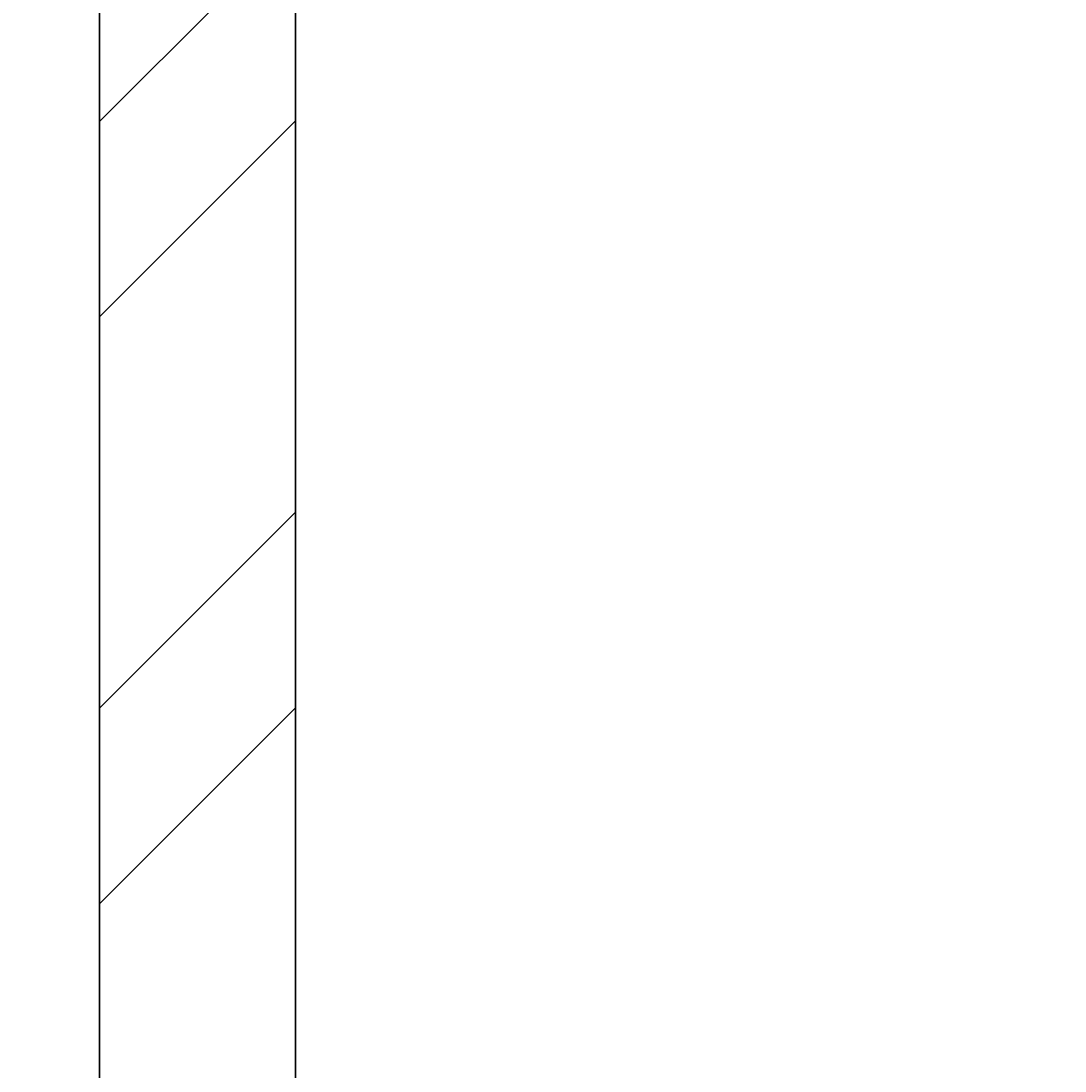
# Model space of a CAD drawing. Units: inches. Extents: x 1885 to 2748, y 783 to 2421.
# Tile 7 of 117: x 1969 to 1993, y 1114 to 1138. Entities that reach past the tile are written whole.
import ezdxf

# ---------------------------------------------------------------- set-up
doc = ezdxf.new("R2010")
doc.units = ezdxf.units.IN
doc.layers.add('A-ANNO-DIMS', color=2, linetype='Continuous', lineweight=18)
doc.layers.add('A-WALL', color=7, linetype='Continuous', lineweight=35)
doc.layers.add('A-WALL-PATT', color=85, linetype='Continuous', lineweight=13, true_color=0x58ba48)
doc.styles.get("Standard").update_dxf_attribs({"font": 'arial.ttf'})
doc.dimstyles.get("Standard").update_dxf_attribs({"dimtxt": 0.18, "dimasz": 0.18, "dimexe": 0.18, "dimexo": 0.0625, "dimgap": 0.09, "dimtad": 0, "dimtih": 1, "dimtoh": 1, "dimdec": 4, "dimzin": 0, "dimdsep": 46, "dimtxsty": 'Standard', "dimcen": 0.09, "dimadec": 0, "dimazin": 0, "dimtfac": 1, "dimtdec": 4, "dimtofl": 0, "dimtmove": 0, "dimatfit": 3, "dimfxl": 1, "dimtolj": 1, "dimtzin": 0, "dimarcsym": 0})

# ---------------------------------------------------------------- blocks, each defined once
blk = doc.blocks.new('*D45')
at = {"layer": 'A-ANNO-DIMS', "color": 0, "lineweight": -2, "transparency": 16777216}
for p, q in [((1980.711, 1524.006), (1902.844, 1524.006)), ((1903.024, 1523.826), (1903.024, 1290.937)), ((1903.024, 1057.686), (1903.024, 1290.574)), ((1971.211, 1057.506), (1902.844, 1057.506))]:
    blk.add_line(p, q, dxfattribs=at)
at = {"layer": 'A-ANNO-DIMS', "color": 0, "transparency": 16777216}
for points in [[(1902.994, 1523.826), (1903.054, 1523.826), (1903.024, 1524.006)], [(1902.994, 1057.686), (1903.054, 1057.686), (1903.024, 1057.506)]]:
    blk.add_solid(points, dxfattribs=at)
at = {"layer": 'Defpoints', "color": 0, "transparency": 16777216}
for p in [(1903.024, 1524.006), (1980.774, 1524.006), (1971.274, 1057.506)]:
    blk.add_point(p, dxfattribs=at)
at = {"layer": 'A-ANNO-DIMS', "color": 0, "transparency": 16777216, "insert": (1903.024, 1290.756), "char_height": 0.18, "attachment_point": 5}
blk.add_mtext('\\A1;466.5', dxfattribs=at)

msp = doc.modelspace()

# ---------------------------------------------------------------- hatches: boundary and pattern name
at = {"layer": 'A-WALL-PATT'}
h = msp.add_hatch(dxfattribs=at)
h.set_pattern_fill('ANSI32', color=256)
h.paths.add_polyline_path([(2007.772, 2318.006), (1980.774, 2318.006), (1980.774, 2281.215), (1985.274, 2281.215), (1985.274, 2313.506), (2007.772, 2313.506), (2007.772, 2315.756)])
h.paths.add_polyline_path([(2094.324, 2318.006), (2067.772, 2318.006), (2067.772, 2313.506), (2094.324, 2313.506), (2094.324, 2315.756)])
h.paths.add_polyline_path([(2131.367, 2315.756), (2131.367, 2318.006), (2131.189, 2318.006), (2112.609, 2318.006), (2112.609, 2313.506), (2117.274, 2313.506), (2117.274, 2255.201), (2121.774, 2255.201), (2121.774, 2313.506), (2131.367, 2313.506)])
h.paths.add_polyline_path([(2190.512, 2318.006), (2155.367, 2318.006), (2155.367, 2313.506), (2169.774, 2313.506), (2169.774, 2229.506), (2121.774, 2229.506), (2121.774, 2233.451), (2119.524, 2233.451), (2117.274, 2233.451), (2117.274, 2201.101), (2121.774, 2201.101), (2121.774, 2225.006), (2169.774, 2225.006), (2169.774, 2165.006), (2306.274, 2165.006), (2306.274, 2066.006), (2310.774, 2066.006), (2344.274, 2066.006), (2486.274, 2066.006), (2486.274, 1886.006), (2483.02, 1886.006), (2483.02, 1881.506), (2486.274, 1881.506), (2486.274, 1880.678), (2490.774, 1880.678), (2490.774, 2070.506), (2344.274, 2070.506), (2310.774, 2070.506), (2310.774, 2165.006), (2310.774, 2173.636), (2308.524, 2173.636), (2306.274, 2173.636), (2306.274, 2169.506), (2174.274, 2169.506), (2174.274, 2313.506), (2190.512, 2313.506), (2190.512, 2315.756)])
h.paths.add_polyline_path([(1985.274, 2221.215), (1980.774, 2221.215), (1980.774, 2165.006), (1992.774, 2165.006), (1992.774, 2141.927), (1997.274, 2141.927), (1997.274, 2165.006), (2117.274, 2165.006), (2117.274, 2163.126), (2121.774, 2163.126), (2121.774, 2172.734), (2119.524, 2172.734), (2117.274, 2172.734), (2117.274, 2169.506), (1985.274, 2169.506)])
h.paths.add_polyline_path([(1997.274, 2105.927), (1992.774, 2105.927), (1992.774, 2070.506), (2016.774, 2070.506), (2016.774, 2059.123), (2019.024, 2059.123), (2021.274, 2059.123), (2021.274, 2070.506), (2117.274, 2070.506), (2117.274, 2022.506), (2114.423, 2022.506), (2114.423, 2018.006), (2123.627, 2018.006), (2123.627, 2020.256), (2123.627, 2022.506), (2121.774, 2022.506), (2121.774, 2142.587), (2119.524, 2142.587), (2117.274, 2142.587), (2117.274, 2075.006), (1997.274, 2075.006)])
h.paths.add_polyline_path([(2092.029, 2020.256), (2092.029, 2022.506), (2021.274, 2022.506), (2021.274, 2035.123), (2016.774, 2035.123), (2016.774, 2018.006), (2016.774, 1978.784), (2021.274, 1978.784), (2021.274, 2018.006), (2092.029, 2018.006)])
h.paths.add_polyline_path([(2260.938, 2022.506), (2153.105, 2022.506), (2153.105, 2020.256), (2153.105, 2018.006), (2155.274, 2018.006), (2155.274, 1886.006), (2107.629, 1886.006), (2107.629, 1881.506), (2182.911, 1881.506), (2182.911, 1883.756), (2182.911, 1886.006), (2159.774, 1886.006), (2159.774, 2018.006), (2260.938, 2018.006), (2260.938, 2020.256)])
h.paths.add_polyline_path([(2047.629, 1883.756), (2047.629, 1886.006), (2021.274, 1886.006), (2021.274, 1918.784), (2019.024, 1918.784), (2016.774, 1918.784), (2016.774, 1881.506), (2047.629, 1881.506)])
h.paths.add_polyline_path([(2306.361, 1883.756), (2306.361, 1886.006), (2296.274, 1886.006), (2296.274, 1982.006), (2316.535, 1982.006), (2316.535, 1984.256), (2316.535, 1986.506), (2296.274, 1986.506), (2296.274, 2022.506), (2289.276, 2022.506), (2289.276, 2018.006), (2291.774, 2018.006), (2291.774, 1886.006), (2242.911, 1886.006), (2242.911, 1881.506), (2306.361, 1881.506)], flags=17)
h.paths.add_polyline_path([(1985.274, 1843.006), (2021.6, 1843.006), (2021.534, 1845.441), (2021.477, 1847.506), (1980.774, 1847.506), (1980.774, 1809.446), (1985.274, 1809.446)])
h.paths.add_polyline_path([(2131.482, 1845.256), (2131.482, 1847.506), (2081.534, 1847.506), (2081.534, 1843.006), (2117.274, 1843.006), (2117.274, 1784.147), (2119.524, 1784.147), (2121.774, 1784.147), (2121.774, 1843.006), (2131.482, 1843.006)])
h.paths.add_polyline_path([(2203.886, 1847.506), (2155.482, 1847.506), (2155.482, 1843.006), (2169.774, 1843.006), (2169.774, 1759.006), (2121.774, 1759.006), (2121.774, 1761.457), (2117.274, 1761.457), (2117.274, 1730.429), (2121.774, 1730.429), (2121.774, 1754.506), (2177.421, 1754.506), (2177.421, 1756.756), (2177.421, 1759.006), (2174.274, 1759.006), (2174.274, 1843.006), (2203.886, 1843.006)])
h.paths.add_polyline_path([(2335.554, 1845.256), (2335.554, 1847.506), (2239.886, 1847.506), (2239.886, 1843.006), (2306.274, 1843.006), (2306.274, 1759.006), (2199.486, 1759.006), (2199.486, 1754.506), (2310.774, 1754.506), (2310.774, 1843.006), (2335.554, 1843.006)])
h.paths.add_polyline_path([(2348.774, 2022.506), (2344.274, 2022.506), (2344.274, 1986.506), (2341.681, 1986.506), (2341.681, 1982.006), (2344.274, 1982.006), (2344.274, 1886.006), (2330.361, 1886.006), (2330.361, 1881.506), (2361.627, 1881.506), (2361.627, 1883.756), (2361.627, 1886.006), (2348.774, 1886.006)], flags=17)
h.paths.add_polyline_path([(2283.251, 2315.756), (2283.251, 2318.006), (2238.512, 2318.006), (2238.512, 2313.506), (2283.251, 2313.506)], flags=17)
h.paths.add_polyline_path([(2363.274, 2348.006), (2388.677, 2348.006), (2388.677, 2350.256), (2388.677, 2352.506), (2358.774, 2352.506), (2358.774, 2348.006), (2358.774, 2318.006), (2344.481, 2318.006), (2344.481, 2313.506), (2358.774, 2313.506), (2358.774, 2229.506), (2310.774, 2229.506), (2310.774, 2231.952), (2306.274, 2231.952), (2306.274, 2205.611), (2310.774, 2205.611), (2310.774, 2225.006), (2358.774, 2225.006), (2358.774, 2211.506), (2452.329, 2211.506), (2452.329, 2213.756), (2452.329, 2216.006), (2363.274, 2216.006), (2363.274, 2318.006)])
h.paths.add_polyline_path([(2310.774, 2313.506), (2320.481, 2313.506), (2320.481, 2315.756), (2320.481, 2318.006), (2302.728, 2318.006), (2302.728, 2313.506), (2306.274, 2313.506), (2306.274, 2251.076), (2310.774, 2251.076)], flags=17)
h.paths.add_polyline_path([(2490.774, 2352.506), (2486.274, 2352.506), (2448.677, 2352.506), (2448.677, 2348.006), (2486.274, 2348.006), (2486.274, 2318.006), (2486.274, 2216.006), (2481.78, 2216.006), (2481.78, 2211.506), (2486.274, 2211.506), (2486.274, 2165.006), (2493.289, 2165.006), (2493.289, 2167.256), (2493.289, 2169.506), (2490.774, 2169.506), (2490.774, 2313.506), (2494.429, 2313.506), (2494.429, 2318.006), (2490.774, 2318.006)])
h.paths.add_polyline_path([(2534.653, 2318.006), (2515.691, 2318.006), (2515.691, 2313.506), (2534.653, 2313.506), (2534.653, 2315.756)])
h.paths.add_polyline_path([(2618.274, 2318.006), (2594.653, 2318.006), (2594.653, 2313.506), (2613.774, 2313.506), (2613.774, 2281.706), (2618.274, 2281.706)])
h.paths.add_polyline_path([(2618.274, 2221.706), (2613.774, 2221.706), (2613.774, 2169.506), (2554.019, 2169.506), (2554.019, 2165.006), (2613.774, 2165.006), (2613.774, 2152.878), (2618.274, 2152.878)])
h.paths.add_polyline_path([(2618.274, 2128.878), (2616.024, 2128.878), (2613.774, 2128.878), (2613.774, 2117.006), (2529.774, 2117.006), (2529.774, 2165.006), (2532.848, 2165.006), (2532.848, 2169.506), (2522.867, 2169.506), (2522.867, 2165.006), (2525.274, 2165.006), (2525.274, 2117.006), (2525.274, 2112.506), (2525.274, 2108.576), (2529.774, 2108.576), (2529.774, 2112.506), (2613.774, 2112.506), (2613.774, 2080.19), (2618.274, 2080.19)])
h.paths.add_polyline_path([(2618.274, 2044.19), (2616.024, 2044.19), (2613.774, 2044.19), (2613.774, 2015.506), (2529.774, 2015.506), (2529.774, 2088.582), (2527.524, 2088.582), (2525.274, 2088.582), (2525.274, 2011.006), (2613.774, 2011.006), (2613.774, 1956.755), (2618.274, 1956.755)])
h.paths.add_polyline_path([(2618.274, 1881.506), (2618.274, 1896.755), (2613.774, 1896.755), (2613.774, 1881.506), (2613.774, 1847.506), (2592.715, 1847.506), (2592.715, 1843.006), (2613.774, 1843.006), (2613.774, 1765.006), (2613.774, 1760.506), (2609.621, 1760.506), (2609.621, 1756.006), (2613.774, 1756.006), (2613.774, 1660.006), (2608.544, 1660.006), (2608.544, 1655.506), (2613.774, 1655.506), (2613.774, 1508.158), (2618.274, 1508.158)])
h.paths.add_polyline_path([(2565.774, 1843.006), (2568.997, 1843.006), (2568.997, 1847.506), (2490.774, 1847.506), (2490.774, 1849.7), (2488.524, 1849.7), (2486.274, 1849.7), (2486.274, 1847.506), (2477.274, 1847.506), (2477.274, 1838.506), (2477.274, 1821.493), (2486.274, 1821.493), (2486.274, 1838.506), (2561.274, 1838.506), (2561.274, 1765.006), (2486.274, 1765.006), (2486.274, 1786.157), (2477.274, 1786.157), (2477.274, 1765.006), (2477.274, 1756.006), (2486.274, 1756.006), (2565.774, 1756.006), (2585.621, 1756.006), (2585.621, 1758.256), (2585.621, 1760.506), (2565.774, 1760.506), (2565.774, 1765.006)])
h.paths.add_polyline_path([(2486.274, 1651.006), (2561.274, 1651.006), (2561.274, 1567.006), (2486.274, 1567.006), (2486.274, 1591.321), (2477.274, 1591.321), (2477.274, 1567.006), (2477.274, 1558.006), (2477.274, 1555.439), (2481.774, 1555.439), (2481.774, 1558.006), (2568.653, 1558.006), (2568.653, 1560.256), (2568.653, 1562.506), (2565.774, 1562.506), (2565.774, 1655.506), (2584.544, 1655.506), (2584.544, 1657.756), (2584.544, 1660.006), (2565.774, 1660.006), (2486.274, 1660.006), (2477.274, 1660.006), (2477.274, 1651.006), (2477.274, 1632.989), (2486.274, 1632.989)])
h.paths.add_polyline_path([(2449.967, 1883.756), (2449.967, 1886.006), (2421.627, 1886.006), (2421.627, 1881.506), (2449.967, 1881.506)], flags=17)
h.paths.add_polyline_path([(2447.274, 1847.506), (2395.554, 1847.506), (2395.554, 1843.006), (2442.774, 1843.006), (2442.774, 1809.27), (2447.274, 1809.27)])
h.paths.add_polyline_path([(1985.274, 1749.446), (1980.774, 1749.446), (1980.774, 1694.504), (1985.274, 1694.504), (1985.274, 1694.506), (1986.897, 1694.506), (1986.897, 1697.78), (1986.897, 1699.006), (1985.274, 1699.006)])
h.paths.add_polyline_path([(2152.774, 1699.006), (2121.774, 1699.006), (2121.774, 1703.668), (2119.524, 1703.668), (2117.274, 1703.668), (2117.274, 1699.006), (2009.219, 1699.006), (2009.219, 1694.506), (2148.274, 1694.506), (2148.274, 1692.631), (2152.774, 1692.631)])
h.paths.add_polyline_path([(2016.274, 1694.506), (2011.774, 1694.506), (2011.774, 1558.006), (2040.806, 1558.006), (2040.806, 1560.256), (2040.806, 1562.506), (2016.274, 1562.506)])
h.paths.add_polyline_path([(2152.774, 1663.017), (2150.524, 1663.017), (2148.274, 1663.017), (2148.274, 1562.506), (2100.806, 1562.506), (2100.806, 1558.006), (2165.119, 1558.006), (2165.119, 1560.256), (2165.119, 1562.506), (2152.774, 1562.506), (2152.774, 1610.506), (2224.774, 1610.506), (2224.774, 1607.99), (2229.274, 1607.99), (2229.274, 1615.006), (2152.774, 1615.006)])
h.paths.add_polyline_path([(2238.613, 1560.256), (2238.613, 1562.506), (2229.274, 1562.506), (2229.274, 1588.756), (2227.024, 1588.763), (2224.774, 1588.771), (2224.774, 1562.506), (2189.119, 1562.506), (2189.119, 1558.006), (2238.613, 1558.006)])
h.paths.add_polyline_path([(2336.024, 1560.256), (2336.024, 1562.506), (2310.774, 1562.506), (2310.774, 1656.347), (2308.524, 1656.347), (2306.274, 1656.347), (2306.274, 1562.506), (2286.613, 1562.506), (2286.613, 1558.006), (2336.024, 1558.006)])
h.paths.add_polyline_path([(2447.274, 1690.968), (2445.024, 1690.968), (2442.774, 1690.968), (2442.774, 1687.006), (2306.274, 1687.006), (2306.274, 1680.75), (2310.774, 1680.75), (2310.774, 1682.506), (2442.774, 1682.506), (2442.774, 1562.506), (2396.024, 1562.506), (2396.024, 1558.006), (2447.274, 1558.006)])
h.paths.add_polyline_path([(2447.274, 1749.27), (2445.024, 1749.27), (2442.774, 1749.27), (2442.774, 1717.232), (2447.274, 1717.232)])
h.paths.add_polyline_path([(2044.674, 1521.756), (2044.674, 1524.006), (2007.274, 1524.006), (2007.274, 1503.49), (2009.524, 1503.49), (2011.774, 1503.49), (2011.774, 1519.506), (2044.674, 1519.506)])
h.paths.add_polyline_path([(2177.969, 1521.756), (2177.969, 1524.006), (2104.674, 1524.006), (2104.674, 1519.506), (2145.774, 1519.506), (2145.774, 1387.506), (2143.37, 1387.506), (2143.37, 1383.006), (2251.585, 1383.006), (2251.585, 1385.256), (2251.585, 1387.506), (2150.274, 1387.506), (2150.274, 1519.506), (2177.969, 1519.506)])
h.paths.add_polyline_path([(2298.704, 1524.006), (2237.969, 1524.006), (2237.969, 1519.506), (2282.274, 1519.506), (2282.274, 1387.506), (2279.683, 1387.506), (2279.683, 1383.006), (2286.774, 1383.006), (2286.774, 1419.006), (2312.451, 1419.006), (2312.451, 1421.256), (2312.451, 1423.506), (2286.774, 1423.506), (2286.774, 1519.506), (2298.704, 1519.506), (2298.704, 1521.722)], flags=17)
h.paths.add_polyline_path([(2361.897, 1521.756), (2361.897, 1524.006), (2322.704, 1524.006), (2322.704, 1519.506), (2334.774, 1519.506), (2334.774, 1423.506), (2331.93, 1423.506), (2331.93, 1419.006), (2334.774, 1419.006), (2334.774, 1387.506), (2334.774, 1383.228), (2339.274, 1383.228), (2339.274, 1387.506), (2339.274, 1519.506), (2361.897, 1519.506)], flags=17)
h.paths.add_polyline_path([(2447.274, 1521.756), (2447.274, 1524.006), (2421.897, 1524.006), (2421.897, 1519.506), (2447.274, 1519.506)], flags=17)
h.paths.add_polyline_path([(2481.774, 1529.6), (2479.524, 1529.6), (2477.274, 1529.6), (2477.274, 1524.006), (2474.489, 1524.006), (2474.489, 1519.506), (2477.274, 1519.506), (2477.274, 1334.506), (2296.774, 1334.506), (2296.774, 1240.506), (2160.274, 1240.506), (2160.274, 1180.506), (2112.274, 1180.506), (2112.274, 1207.692), (2110.024, 1207.692), (2107.774, 1207.692), (2107.774, 1171.609), (2112.274, 1171.609), (2112.274, 1176.006), (2160.274, 1176.006), (2160.274, 1092.006), (2144.221, 1092.006), (2144.221, 1087.506), (2189.497, 1087.506), (2189.497, 1089.756), (2189.497, 1092.006), (2164.774, 1092.006), (2164.774, 1236.006), (2296.774, 1236.006), (2296.774, 1231.912), (2301.274, 1231.912), (2301.274, 1330.006), (2481.774, 1330.006), (2481.774, 1387.506)])
h.paths.add_polyline_path([(2618.274, 1448.158), (2613.774, 1448.158), (2613.774, 1382.506), (2529.774, 1382.506), (2525.274, 1382.506), (2525.274, 1307.062), (2529.774, 1307.062), (2529.774, 1378.006), (2613.774, 1378.006), (2613.774, 1354.988), (2618.274, 1354.988)])
h.paths.add_polyline_path([(2618.274, 1318.988), (2613.774, 1318.988), (2613.774, 1281.006), (2529.774, 1281.006), (2529.774, 1283.786), (2527.524, 1283.786), (2525.274, 1283.786), (2525.274, 1228.506), (2516.794, 1228.506), (2516.794, 1224.006), (2533.484, 1224.006), (2533.484, 1226.256), (2533.484, 1228.506), (2529.774, 1228.506), (2529.774, 1276.506), (2613.774, 1276.506), (2613.774, 1266.02), (2618.274, 1266.02)])
h.paths.add_polyline_path([(2618.274, 1134.964), (2613.774, 1134.964), (2613.774, 1092.006), (2594.545, 1092.006), (2594.545, 1087.506), (2618.274, 1087.506)])
h.paths.add_polyline_path([(2534.545, 1092.006), (2509.765, 1092.006), (2509.765, 1087.506), (2534.545, 1087.506), (2534.545, 1089.756)])
h.paths.add_polyline_path([(2481.274, 1224.006), (2484.117, 1224.006), (2484.117, 1226.256), (2484.117, 1228.506), (2476.774, 1228.506), (2476.774, 1198.506), (2471.61, 1198.506), (2471.61, 1194.006), (2476.774, 1194.006), (2476.774, 1062.006), (2436.894, 1062.006), (2436.894, 1057.506), (2476.774, 1057.506), (2481.274, 1057.506), (2481.274, 1062.006), (2481.274, 1087.506), (2485.354, 1087.506), (2485.354, 1089.756), (2485.354, 1092.006), (2481.274, 1092.006), (2481.274, 1117.506)])
h.paths.add_polyline_path([(2439.898, 1198.506), (2349.274, 1198.506), (2349.274, 1194.006), (2349.274, 1180.506), (2301.274, 1180.506), (2301.274, 1201.896), (2299.024, 1201.896), (2296.774, 1201.896), (2296.774, 1172.335), (2299.024, 1172.335), (2301.274, 1172.335), (2301.274, 1176.006), (2349.274, 1176.006), (2349.274, 1092.006), (2334.452, 1092.006), (2334.452, 1087.506), (2349.274, 1087.506), (2349.274, 1057.506), (2353.774, 1057.506), (2376.894, 1057.506), (2376.894, 1059.756), (2376.894, 1062.006), (2353.774, 1062.006), (2353.774, 1087.506), (2353.774, 1180.506), (2353.774, 1194.006), (2439.898, 1194.006), (2439.898, 1196.256)])
h.paths.add_polyline_path([(2270.596, 1089.756), (2270.596, 1092.006), (2249.497, 1092.006), (2249.497, 1087.506), (2270.596, 1087.506)], flags=17)
h.paths.add_polyline_path([(2310.452, 1092.006), (2301.274, 1092.006), (2301.274, 1153.292), (2296.774, 1153.292), (2296.774, 1092.006), (2293.786, 1092.006), (2293.786, 1087.506), (2310.452, 1087.506), (2310.452, 1089.756)], flags=17)
h.paths.add_polyline_path([(2112.274, 1150.328), (2110.024, 1150.328), (2107.774, 1150.328), (2107.774, 1092.006), (2104.465, 1092.006), (2104.465, 1087.506), (2120.221, 1087.506), (2120.221, 1089.756), (2120.221, 1092.006), (2112.274, 1092.006)])
h.paths.add_polyline_path([(2082.172, 1092.006), (2058.144, 1092.006), (2058.144, 1087.506), (2082.172, 1087.506), (2082.172, 1089.756)])
h.paths.add_polyline_path([(1975.774, 1145.638), (1971.274, 1145.638), (1971.274, 1087.506), (1980.774, 1087.506), (1998.144, 1087.506), (1998.144, 1089.756), (1998.144, 1092.006), (1985.274, 1092.006), (1975.774, 1092.006)])
h.paths.add_polyline_path([(2112.274, 1244.385), (2110.024, 1244.385), (2107.774, 1244.385), (2107.774, 1240.506), (1992.274, 1240.506), (1992.274, 1271.008), (1987.774, 1271.008), (1987.774, 1240.506), (1980.774, 1240.506), (1975.774, 1240.506), (1971.274, 1240.506), (1971.274, 1205.638), (1975.774, 1205.638), (1975.774, 1236.006), (2107.774, 1236.006), (2107.774, 1233.444), (2112.274, 1233.444), (2112.274, 1236.006)])
h.paths.add_polyline_path([(2112.274, 1383.006), (2114.783, 1383.006), (2114.783, 1385.256), (2114.783, 1387.506), (2102.476, 1387.506), (2102.476, 1383.006), (2107.774, 1383.006), (2107.774, 1335.006), (2011.774, 1335.006), (2011.774, 1349.939), (2007.274, 1349.939), (2007.274, 1335.006), (1987.774, 1335.006), (1987.774, 1330.506), (1987.774, 1307.008), (1992.274, 1307.008), (1992.274, 1330.506), (2007.274, 1330.506), (2107.774, 1330.506), (2107.774, 1264.711), (2112.274, 1264.711)])
h.paths.add_polyline_path([(2077.857, 1387.506), (2011.774, 1387.506), (2011.774, 1390.036), (2009.524, 1390.036), (2007.274, 1390.036), (2007.274, 1373.939), (2011.774, 1373.939), (2011.774, 1383.006), (2077.857, 1383.006)])
h.paths.add_polyline_path([(2011.774, 1443.49), (2007.274, 1443.49), (2007.274, 1410.248), (2011.774, 1410.248)])

# ---------------------------------------------------------------- linework, layer by layer
at = {"layer": 'A-WALL'}
for p, q in [((1971.274, 1145.638), (1971.274, 1087.506)), ((1975.774, 1145.638), (1975.774, 1092.006))]:
    msp.add_line(p, q, dxfattribs=at)

# ---------------------------------------------------------------- dimensions: what is measured, and where the dimension line sits
at = {"layer": 'A-ANNO-DIMS'}
dim = msp.add_linear_dim(base=(1903.024, 1524.006), p1=(1971.274, 1057.506), p2=(1980.774, 1524.006), angle=90, dimstyle='Standard', override={"dimdec": 1, "dimlfac": 1, "dimrnd": 0, "dimzin": 0, "dimdsep": 46, "dimlunit": 2}, dxfattribs=at)
dim.commit()
dim.dimension.update_dxf_attribs({"geometry": '*D45', "text_midpoint": (1903.024, 1290.756)})

doc.saveas('drawing.dxf')
